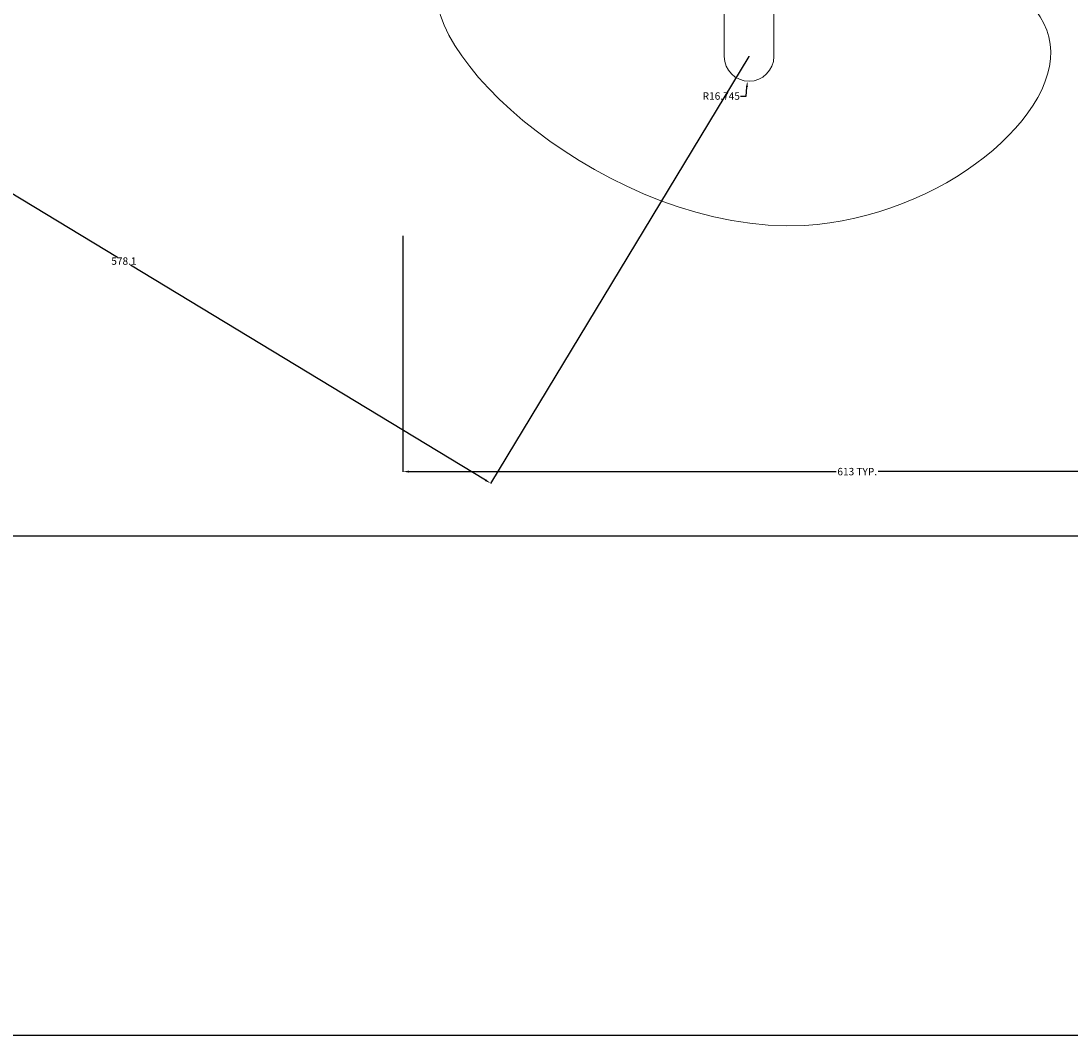
# Model space of a CAD drawing. Units: metres. Extents: x -2391 to 4922, y -635 to 4845.
# Tile 5 of 37: x -1367 to -659, y -635 to 53. Entities that reach past the tile are written whole.
import ezdxf

# ---------------------------------------------------------------- set-up
doc = ezdxf.new("R2010")
doc.units = ezdxf.units.M
doc.header["$MEASUREMENT"] = 0
doc.layers.add('A-ANNO-DIMS', color=2, linetype='Continuous', lineweight=18)
doc.layers.add('A-FURN', color=8, linetype='Continuous', lineweight=18)
doc.styles.get("Standard").update_dxf_attribs({"font": 'arial.ttf'})
doc.dimstyles.get("Standard").update_dxf_attribs({"dimtxt": 5, "dimasz": 4, "dimexe": 0.18, "dimexo": 0.0625, "dimgap": 0.09, "dimtad": 0, "dimtih": 1, "dimtoh": 1, "dimdec": 0, "dimzin": 0, "dimdsep": 46, "dimtxsty": 'Standard', "dimcen": 0.09, "dimadec": 0, "dimazin": 0, "dimtfac": 1, "dimtdec": 0, "dimtofl": 0, "dimtmove": 0, "dimatfit": 3, "dimfxl": 1, "dimtolj": 1, "dimtzin": 0, "dimarcsym": 0})

# ---------------------------------------------------------------- blocks, each defined once
blk = doc.blocks.new('STOOL-BAR')
for p, q in [((227.15, 541.57), (227.15, 114.21)), ((193.66, 114.21), (193.66, 537.32))]:
    blk.add_line(p, q)
blk.add_arc((210.41, 114.21), 16.75, 180, 0)
blk.add_open_spline([(193.66, 199.14), (106.89, 200.34), (-113.88, 203.37), (215.44, -95.9), (508.37, 143.53), (296.52, 208.79), (227.15, 200.77)], degree=3, knots=[0, 0, 0, 0, 131.596892, 334.838301, 476.929251, 613.088937, 613.088937, 613.088937, 613.088937])
blk = doc.blocks.new('*D7')
at = {"layer": 'A-ANNO-DIMS', "color": 0, "lineweight": -2, "transparency": 16777216}
for p, q in [((-1109.41, -92.24), (-1109.41, -251.4)), ((-496.6, -92.24), (-496.6, -251.4)), ((-1105.41, -251.22), (-817.22, -251.22)), ((-500.6, -251.22), (-788.79, -251.22))]:
    blk.add_line(p, q, dxfattribs=at)
at = {"layer": 'A-ANNO-DIMS', "color": 0, "transparency": 16777216}
for points in [[(-1105.41, -250.56), (-1105.41, -251.89), (-1109.41, -251.22)], [(-500.6, -250.56), (-500.6, -251.89), (-496.6, -251.22)]]:
    blk.add_solid(points, dxfattribs=at)
at = {"layer": 'Defpoints', "color": 0, "transparency": 16777216}
for p in [(-1109.41, -92.18), (-496.6, -92.18), (-496.6, -251.22)]:
    blk.add_point(p, dxfattribs=at)
at = {"layer": 'A-ANNO-DIMS', "color": 0, "transparency": 16777216, "insert": (-803, -251.22), "char_height": 5, "attachment_point": 5}
blk.add_mtext('\\A1;613 TYP.', dxfattribs=at)
blk = doc.blocks.new('*D8')
at = {"layer": 'A-ANNO-DIMS', "color": 0, "lineweight": -2, "transparency": 16777216}
for p, q in [((-2047.33, 3005.21), (-2047.33, -631.4)), ((4577.76, 2350.21), (4577.76, -631.4)), ((-2043.33, -631.22), (1257.62, -631.22)), ((4573.76, -631.22), (1272.8, -631.22))]:
    blk.add_line(p, q, dxfattribs=at)
at = {"layer": 'A-ANNO-DIMS', "color": 0, "transparency": 16777216}
for points in [[(-2043.33, -630.56), (-2043.33, -631.89), (-2047.33, -631.22)], [(4573.76, -630.56), (4573.76, -631.89), (4577.76, -631.22)]]:
    blk.add_solid(points, dxfattribs=at)
at = {"layer": 'Defpoints', "color": 0, "transparency": 16777216}
for p in [(-2047.33, 3005.28), (4577.76, 2350.28), (4577.76, -631.22)]:
    blk.add_point(p, dxfattribs=at)
at = {"layer": 'A-ANNO-DIMS', "color": 0, "transparency": 16777216, "insert": (1265.21, -631.22), "char_height": 5, "attachment_point": 5}
blk.add_mtext('\\A1;6625', dxfattribs=at)
blk = doc.blocks.new('*D10')
at = {"layer": 'A-ANNO-DIMS', "color": 0, "lineweight": -2, "transparency": 16777216}
for p, q in [((550.68, 4505.28), (-2384.01, 4505.28)), ((-2383.83, 4501.28), (-2383.83, 2107.92)), ((-2383.83, -290.72), (-2383.83, 2102.63)), ((-488.55, -294.72), (-2384.01, -294.72))]:
    blk.add_line(p, q, dxfattribs=at)
at = {"layer": 'A-ANNO-DIMS', "color": 0, "transparency": 16777216}
for points in [[(-2384.5, 4501.28), (-2383.17, 4501.28), (-2383.83, 4505.28)], [(-2384.5, -290.72), (-2383.17, -290.72), (-2383.83, -294.72)]]:
    blk.add_solid(points, dxfattribs=at)
at = {"layer": 'Defpoints', "color": 0, "transparency": 16777216}
for p in [(-2383.83, 4505.28), (550.74, 4505.28), (-488.49, -294.72)]:
    blk.add_point(p, dxfattribs=at)
at = {"layer": 'A-ANNO-DIMS', "color": 0, "transparency": 16777216, "insert": (-2383.83, 2105.28), "char_height": 5, "attachment_point": 5}
blk.add_mtext('\\A1;4800', dxfattribs=at)
blk = doc.blocks.new('*D51')
at = {"layer": 'A-ANNO-DIMS', "color": 0, "lineweight": -2, "transparency": 16777216}
for p, q in [((-1370.51, 328.28), (-1544.92, 40.37)), ((-1541.41, 38.45), (-1301.95, -106.62)), ((-876.02, 28.72), (-1050.43, -259.19)), ((-1053.76, -256.97), (-1293.22, -111.9))]:
    blk.add_line(p, q, dxfattribs=at)
at = {"layer": 'A-ANNO-DIMS', "color": 0, "transparency": 16777216}
for points in [[(-1541.06, 39.02), (-1541.75, 37.88), (-1544.83, 40.52)], [(-1053.42, -256.39), (-1054.11, -257.54), (-1050.34, -259.04)]]:
    blk.add_solid(points, dxfattribs=at)
at = {"layer": 'Defpoints', "color": 0, "transparency": 16777216}
for p in [(-1370.48, 328.33), (-1544.83, 40.52), (-875.99, 28.77)]:
    blk.add_point(p, dxfattribs=at)
at = {"layer": 'A-ANNO-DIMS', "color": 0, "transparency": 16777216, "insert": (-1297.58, -109.26), "char_height": 5, "attachment_point": 5}
blk.add_mtext('\\A1;578.1', dxfattribs=at)
blk = doc.blocks.new('*D54')
at = {"layer": 'A-ANNO-DIMS', "color": 0, "lineweight": -2, "transparency": 16777216}
for p, q in [((-876.08, 28.77), (-875.9, 28.77)), ((-875.99, 28.68), (-875.99, 28.86)), ((-877.82, 2.04), (-877.41, 8.07)), ((-881.82, 2.04), (-877.82, 2.04))]:
    blk.add_line(p, q, dxfattribs=at)
at = {"layer": 'A-ANNO-DIMS', "color": 0, "transparency": 16777216}
blk.add_solid([(-878.07, 8.12), (-876.74, 8.03), (-877.13, 12.06)], dxfattribs=at)
at = {"layer": 'Defpoints', "color": 0, "transparency": 16777216}
for p in [(-875.99, 28.77), (-877.13, 12.06)]:
    blk.add_point(p, dxfattribs=at)
at = {"layer": 'A-ANNO-DIMS', "color": 0, "transparency": 16777216, "insert": (-894.7, 2.04), "char_height": 5, "attachment_point": 5}
blk.add_mtext('\\A1;R16.745', dxfattribs=at)

msp = doc.modelspace()

# ---------------------------------------------------------------- block references
at = {"layer": 'A-FURN'}
msp.add_blockref('STOOL-BAR', (-1086.3941, -85.4426), dxfattribs=at)

# ---------------------------------------------------------------- dimensions: what is measured, and where the dimension line sits
at = {"layer": 'A-ANNO-DIMS'}
for base, p1, p2, angle, override, picture, middle in [((-2383.8343, 4505.2763), (-488.4886, -294.7237), (550.7419, 4505.2763), 90, {"dimdec": 0, "dimlfac": 1, "dimrnd": 0, "dimzin": 0, "dimdsep": 46, "dimlunit": 2}, '*D10', (-2383.8343, 2105.2763)), ((-1544.828, 40.5209), (-875.9874, 28.7702), (-1370.4753, 328.3288), 148.7927031, {"dimdec": 1, "dimlfac": 1, "dimrnd": 0, "dimzin": 0, "dimdsep": 46, "dimlunit": 2}, '*D51', (-1297.5841, -109.2584))]:
    dim = msp.add_linear_dim(base=base, p1=p1, p2=p2, angle=angle, dimstyle='Standard', override=override, dxfattribs=at)
    dim.commit()
    dim.dimension.update_dxf_attribs({"geometry": picture, "text_midpoint": middle})
dim = msp.add_linear_dim(base=(4577.76, -631.2237), p1=(-2047.3343, 3005.2763), p2=(4577.76, 2350.2763), dimstyle='Standard', override={"dimdec": 0, "dimlfac": 1, "dimrnd": 0, "dimzin": 0, "dimdsep": 46, "dimlunit": 2}, dxfattribs=at)
dim.commit()
dim.dimension.update_dxf_attribs({"geometry": '*D8', "text_midpoint": (1265.2128, -631.2237)})
dim = msp.add_radius_dim(center=(-875.9874, 28.7702), mpoint=(-877.1327, 12.064), dimstyle='Standard', override={"dimdec": 3, "dimlfac": 1, "dimrnd": 0, "dimzin": 0, "dimdsep": 46, "dimlunit": 2}, dxfattribs=at)
dim.commit()
dim.dimension.update_dxf_attribs({"geometry": '*D54', "text_midpoint": (-894.6998, 2.0403), "dimtype": 164})
dim = msp.add_linear_dim(base=(-496.6042, -251.2224), p1=(-1109.4055, -92.1799), p2=(-496.6042, -92.1799), text='<> TYP.', dimstyle='Standard', override={"dimdec": 0, "dimrnd": 0, "dimzin": 0, "dimlunit": 2}, dxfattribs=at)
dim.commit()
dim.dimension.update_dxf_attribs({"geometry": '*D7', "text_midpoint": (-803.0049, -251.2224)})

doc.saveas('drawing.dxf')
